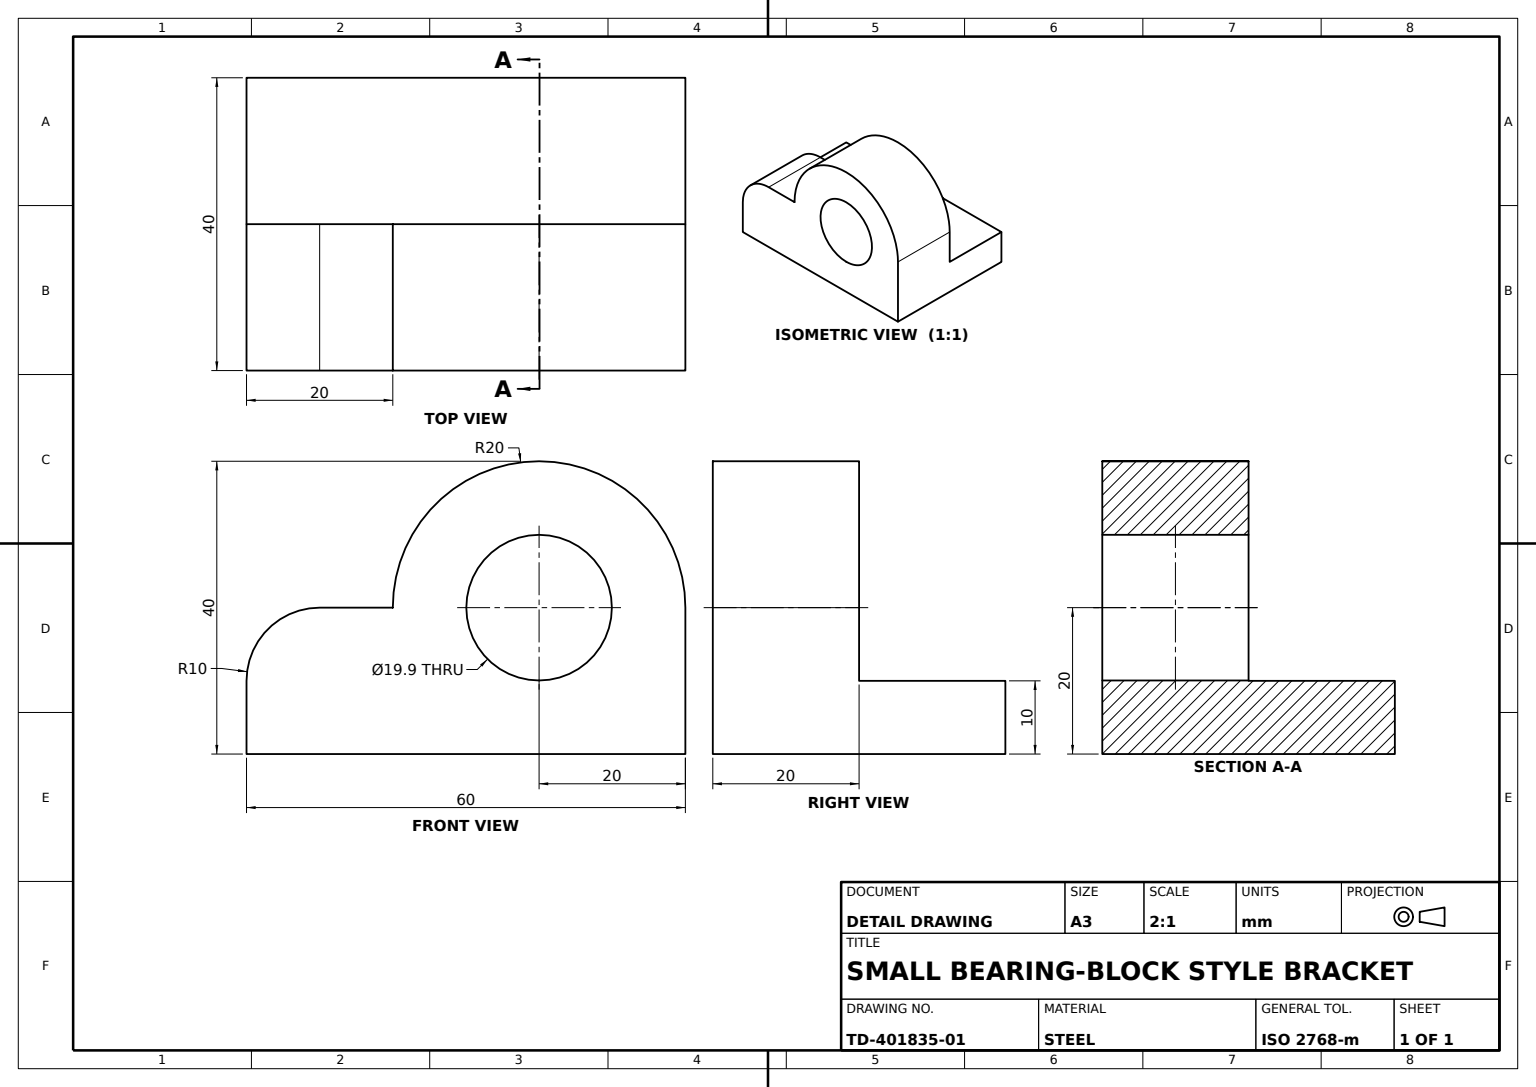
from build123d import *

# Parameters (mm, degrees)
BRACKET_BODY_DEPTH      = 30
BOSS_ROUNDING_SKETCH_R  = 9.95
BOSS_ROUNDING_CUT_DEPTH = 60
BORE_CUT_DEPTH          = 60


with BuildPart() as part:
    # Bracket Profile Sketch → Bracket Body (new, symmetric)
    with BuildSketch(Plane(origin=(0, 0, 0), x_dir=(0, 0, -1), z_dir=(1, 0, 0))):
        Polygon((0, 0), (40, 0), (40, 10), (20, 10), (20, 40), (0, 40), align=None)
    extrude(amount=BRACKET_BODY_DEPTH, both=True)

    # Boss Rounding Sketch → Boss Rounding Cut (cut)
    with BuildSketch(Plane(origin=(0, 0, -20), x_dir=(-1, 0, 0), z_dir=(0, 0, -1))):
        with Locations(Location((-10, 20, 0), (0, 0, 90))):
            Circle(BOSS_ROUNDING_SKETCH_R)
    extrude(amount=-BOSS_ROUNDING_CUT_DEPTH, mode=Mode.SUBTRACT)

    # Bore Sketch → Bore Cut (cut)
    with BuildSketch(Plane(origin=(0, 0, -20), x_dir=(-1, 0, 0), z_dir=(0, 0, -1))):
        with BuildLine():
            ThreePointArc((-30, 20), (-24.142135624, 34.142135624), (-10, 40))
            Line((-10, 40), (-30, 40))
            Line((-30, 40), (-30, 20))
        make_face()
        with BuildLine():
            ThreePointArc((-10, 40), (4.142135624, 34.142135624), (10, 20))
            Line((10, 20), (20, 20))
            ThreePointArc((20, 20), (27.071067812, 17.071067812), (30, 10))
            Line((30, 10), (30, 40))
            Line((30, 40), (-10, 40))
        make_face()
    extrude(amount=-BORE_CUT_DEPTH, mode=Mode.SUBTRACT)


solid = part.part
